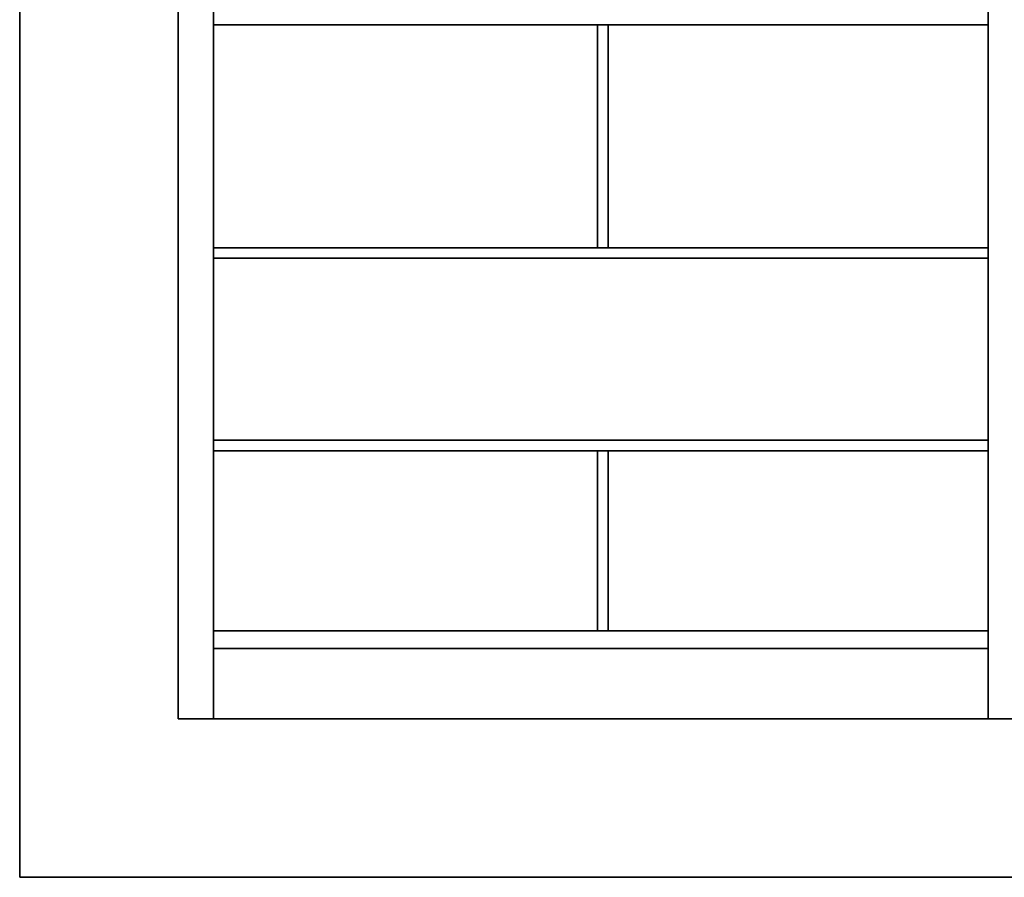
# Model space of a CAD drawing. Units: inches. Extents: x 64 to 1167, y 117 to 939.
# Tile 29 of 56: x 983 to 1039, y 428 to 476. Entities that reach past the tile are written whole.
import ezdxf

# ---------------------------------------------------------------- set-up
doc = ezdxf.new("R2010")
doc.units = ezdxf.units.IN
doc.header["$MEASUREMENT"] = 0
doc.layers.add('A-SECT', color=7, linetype='Continuous', lineweight=35)

msp = doc.modelspace()

# ---------------------------------------------------------------- linework, layer by layer
at = {"layer": 'A-SECT'}
for p, q in [((991.813, 556.679), (991.813, 436.679)), ((993.813, 538.679), (993.813, 436.679)), ((1037.813, 538.679), (1037.813, 436.679)), ((1037.813, 476.079), (993.813, 476.079)), ((1015.631, 476.079), (1015.631, 463.431)), ((1016.231, 476.079), (1016.231, 463.431)), ((1037.813, 463.431), (993.813, 463.431)), ((1037.813, 462.831), (993.813, 462.831)), ((1037.813, 452.501), (993.813, 452.501)), ((1037.813, 451.901), (993.813, 451.901)), ((1015.631, 451.901), (1015.631, 441.679)), ((1016.231, 451.901), (1016.231, 441.679)), ((993.813, 441.679), (1037.813, 441.679)), ((993.813, 440.679), (1037.813, 440.679)), ((991.813, 436.679), (1157.813, 436.679))]:
    msp.add_line(p, q, dxfattribs=at)
msp.add_lwpolyline([(982.813, 427.679), (1166.813, 427.679), (1166.813, 565.679), (982.813, 565.679)], close=True, dxfattribs=at)

doc.saveas('drawing.dxf')
